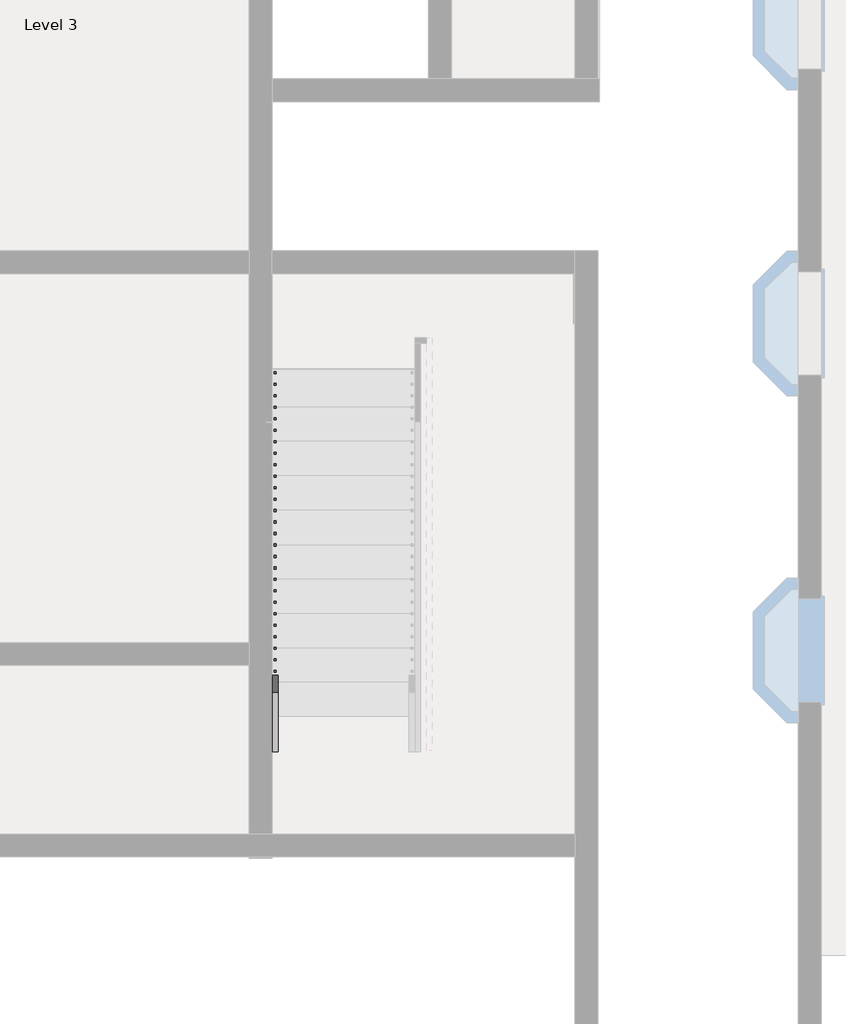
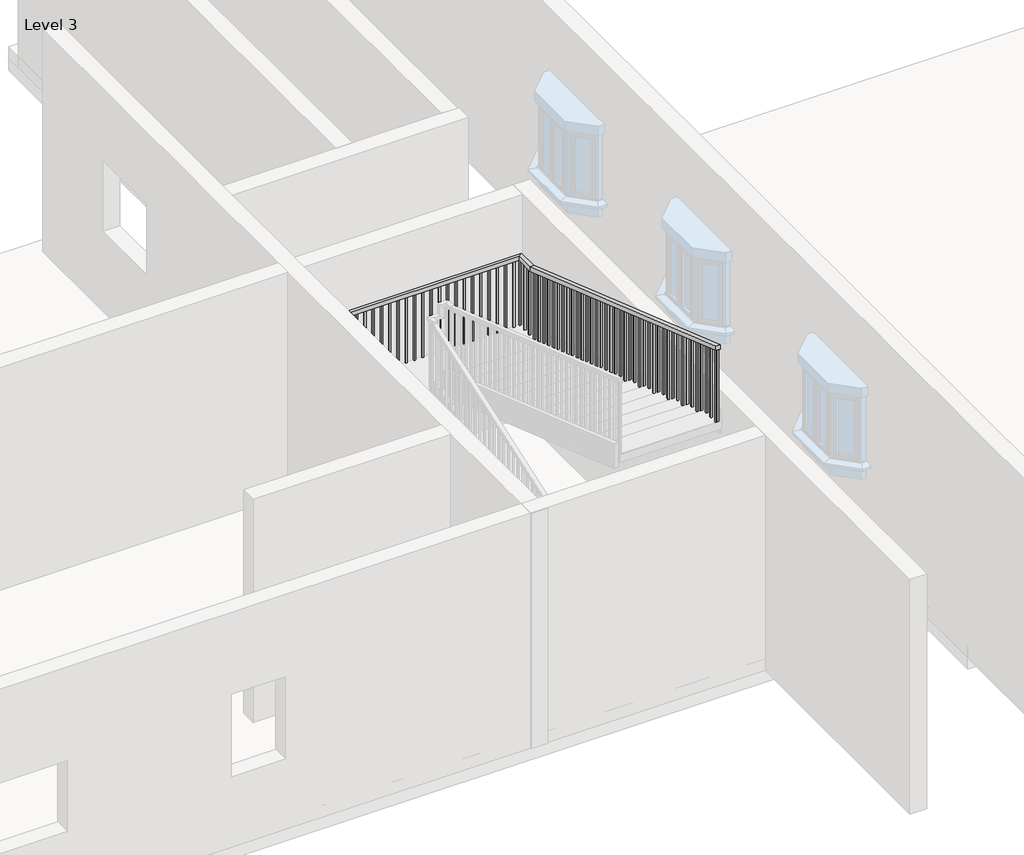
# One storey, part 8 of 14: 1 railing.
"""IFC4 building model written with IfcOpenShell, lengths in millimetres."""

from ifc_helpers import new_model, si_unit, frame, origin, place, context, project, spatial, polyline, outline, extrude, faceted_brep, element, save

model = new_model("IFC4")

# Units and contexts
model_context = context("Model", 3, world=origin())
ifc_project = project(units=[si_unit("LENGTHUNIT", "METRE", prefix="MILLI")], contexts=[model_context])

# Site, building, storey
site = spatial("IfcSite", under=ifc_project)
building = spatial("IfcBuilding", under=site)
storey = spatial("IfcBuildingStorey", under=building, Name="Level 3", Elevation=6096.0)

# Railing
placement = place(None, origin())
element("IfcRailing", 1, ObjectType="Handrail - Rectangular", at=placement, inside=storey, context=model_context, shape_type="SolidModel", body=[
    faceted_brep([(-3857.687215, -9955.5916506, 7115.9076923), (-3857.687215, -9955.5916506, 7062.1602476), (-3806.887215, -9955.5916506, 7062.1602476), (-3806.887215, -9955.5916506, 7115.9076923), (-3857.687215, -6291.6416506, 8382.0), (-3857.687215, -6283.1120276, 8331.2), (-3806.887215, -6283.1120276, 8331.2), (-3806.887215, -6291.6416506, 8382.0), (-3857.687215, -5713.7916506, 8382.0), (-3857.687215, -5713.7916506, 8331.2), (-3806.887215, -5764.5916506, 8331.2), (-3806.887215, -5764.5916506, 8382.0), (-1190.687215, -5713.7916506, 8382.0), (-1190.687215, -5713.7916506, 8331.2), (-1241.487215, -5764.5916506, 8331.2), (-1241.487215, -5764.5916506, 8382.0), (-1190.687215, -5986.8416506, 8382.0), (-1190.687215, -5995.3852679, 8331.2), (-1241.487215, -5995.3852679, 8331.2), (-1241.487215, -5986.8416506, 8382.0), (-1190.687215, -9949.2416506, 9753.6), (-1241.487215, -9949.2416506, 9753.6), (-1241.487215, -9949.2416506, 9699.842594), (-1190.687215, -9949.2416506, 9699.842594)], [[[0, 1, 2, 3]], [[1, 0, 4, 5]], [[2, 1, 5, 6]], [[3, 2, 6, 7]], [[0, 3, 7, 4]], [[5, 4, 8, 9]], [[6, 5, 9, 10]], [[7, 6, 10, 11]], [[4, 7, 11, 8]], [[9, 8, 12, 13]], [[10, 9, 13, 14]], [[11, 10, 14, 15]], [[8, 11, 15, 12]], [[13, 12, 16, 17]], [[14, 13, 17, 18]], [[15, 14, 18, 19]], [[12, 15, 19, 16]], [[20, 21, 22, 23]], [[17, 16, 20, 23]], [[18, 17, 23, 22]], [[19, 18, 22, 21]], [[16, 19, 21, 20]]]),
    extrude(outline(polyline([(-9895.2666506, 9681.1589402), (-9895.2666506, 8733.6923077), (-9914.3166506, 8733.6923077), (-9914.3166506, 9687.7531709), (-9895.2666506, 9681.1589402)])), frame((-1225.612215, 0.0, 0.0), z_axis=(1.0, 0.0, 0.0), x_axis=(0.0, 1.0, 0.0)), (0.0, 0.0, 1.0), 19.05),
    extrude(outline(polyline([(-9793.6666506, 9645.9897094), (-9793.6666506, 8733.6923077), (-9812.7166506, 8733.6923077), (-9812.7166506, 9652.5839402), (-9793.6666506, 9645.9897094)])), frame((-1225.612215, 0.0, 0.0), z_axis=(1.0, 0.0, 0.0), x_axis=(0.0, 1.0, 0.0)), (0.0, 0.0, 1.0), 19.05),
    extrude(outline(polyline([(-9692.0666506, 9610.8204786), (-9692.0666506, 8733.6923077), (-9711.1166506, 8733.6923077), (-9711.1166506, 9617.4147094), (-9692.0666506, 9610.8204786)])), frame((-1225.612215, 0.0, 0.0), z_axis=(1.0, 0.0, 0.0), x_axis=(0.0, 1.0, 0.0)), (0.0, 0.0, 1.0), 19.05),
    extrude(outline(polyline([(-9590.4666506, 9575.6512479), (-9590.4666506, 8628.1846154), (-9609.5166506, 8628.1846154), (-9609.5166506, 9582.2454786), (-9590.4666506, 9575.6512479)])), frame((-1225.612215, 0.0, 0.0), z_axis=(1.0, 0.0, 0.0), x_axis=(0.0, 1.0, 0.0)), (0.0, 0.0, 1.0), 19.05),
    extrude(outline(polyline([(-9488.8666506, 9540.4820171), (-9488.8666506, 8628.1846154), (-9507.9166506, 8628.1846154), (-9507.9166506, 9547.0762479), (-9488.8666506, 9540.4820171)])), frame((-1225.612215, 0.0, 0.0), z_axis=(1.0, 0.0, 0.0), x_axis=(0.0, 1.0, 0.0)), (0.0, 0.0, 1.0), 19.05),
    extrude(outline(polyline([(-9387.2666506, 9505.3127863), (-9387.2666506, 8628.1846154), (-9406.3166506, 8628.1846154), (-9406.3166506, 9511.9070171), (-9387.2666506, 9505.3127863)])), frame((-1225.612215, 0.0, 0.0), z_axis=(1.0, 0.0, 0.0), x_axis=(0.0, 1.0, 0.0)), (0.0, 0.0, 1.0), 19.05),
    extrude(outline(polyline([(-9285.6666506, 9470.1435556), (-9285.6666506, 8522.6769231), (-9304.7166506, 8522.6769231), (-9304.7166506, 9476.7377863), (-9285.6666506, 9470.1435556)])), frame((-1225.612215, 0.0, 0.0), z_axis=(1.0, 0.0, 0.0), x_axis=(0.0, 1.0, 0.0)), (0.0, 0.0, 1.0), 19.05),
    extrude(outline(polyline([(-9184.0666506, 9434.9743248), (-9184.0666506, 8522.6769231), (-9203.1166506, 8522.6769231), (-9203.1166506, 9441.5685556), (-9184.0666506, 9434.9743248)])), frame((-1225.612215, 0.0, 0.0), z_axis=(1.0, 0.0, 0.0), x_axis=(0.0, 1.0, 0.0)), (0.0, 0.0, 1.0), 19.05),
    extrude(outline(polyline([(-9082.4666506, 9399.805094), (-9082.4666506, 8522.6769231), (-9101.5166506, 8522.6769231), (-9101.5166506, 9406.3993248), (-9082.4666506, 9399.805094)])), frame((-1225.612215, 0.0, 0.0), z_axis=(1.0, 0.0, 0.0), x_axis=(0.0, 1.0, 0.0)), (0.0, 0.0, 1.0), 19.05),
    extrude(outline(polyline([(-8980.8666506, 9364.6358632), (-8980.8666506, 8417.1692308), (-8999.9166506, 8417.1692308), (-8999.9166506, 9371.230094), (-8980.8666506, 9364.6358632)])), frame((-1225.612215, 0.0, 0.0), z_axis=(1.0, 0.0, 0.0), x_axis=(0.0, 1.0, 0.0)), (0.0, 0.0, 1.0), 19.05),
    extrude(outline(polyline([(-8879.2666506, 9329.4666325), (-8879.2666506, 8417.1692308), (-8898.3166506, 8417.1692308), (-8898.3166506, 9336.0608632), (-8879.2666506, 9329.4666325)])), frame((-1225.612215, 0.0, 0.0), z_axis=(1.0, 0.0, 0.0), x_axis=(0.0, 1.0, 0.0)), (0.0, 0.0, 1.0), 19.05),
    extrude(outline(polyline([(-8777.6666506, 9294.2974017), (-8777.6666506, 8417.1692308), (-8796.7166506, 8417.1692308), (-8796.7166506, 9300.8916325), (-8777.6666506, 9294.2974017)])), frame((-1225.612215, 0.0, 0.0), z_axis=(1.0, 0.0, 0.0), x_axis=(0.0, 1.0, 0.0)), (0.0, 0.0, 1.0), 19.05),
    extrude(outline(polyline([(-8676.0666506, 9259.1281709), (-8676.0666506, 8311.6615385), (-8695.1166506, 8311.6615385), (-8695.1166506, 9265.7224017), (-8676.0666506, 9259.1281709)])), frame((-1225.612215, 0.0, 0.0), z_axis=(1.0, 0.0, 0.0), x_axis=(0.0, 1.0, 0.0)), (0.0, 0.0, 1.0), 19.05),
    extrude(outline(polyline([(-8574.4666506, 9223.9589402), (-8574.4666506, 8311.6615385), (-8593.5166506, 8311.6615385), (-8593.5166506, 9230.5531709), (-8574.4666506, 9223.9589402)])), frame((-1225.612215, 0.0, 0.0), z_axis=(1.0, 0.0, 0.0), x_axis=(0.0, 1.0, 0.0)), (0.0, 0.0, 1.0), 19.05),
    extrude(outline(polyline([(-8472.8666506, 9188.7897094), (-8472.8666506, 8311.6615385), (-8491.9166506, 8311.6615385), (-8491.9166506, 9195.3839402), (-8472.8666506, 9188.7897094)])), frame((-1225.612215, 0.0, 0.0), z_axis=(1.0, 0.0, 0.0), x_axis=(0.0, 1.0, 0.0)), (0.0, 0.0, 1.0), 19.05),
    extrude(outline(polyline([(-8371.2666506, 9153.6204786), (-8371.2666506, 8206.1538462), (-8390.3166506, 8206.1538462), (-8390.3166506, 9160.2147094), (-8371.2666506, 9153.6204786)])), frame((-1225.612215, 0.0, 0.0), z_axis=(1.0, 0.0, 0.0), x_axis=(0.0, 1.0, 0.0)), (0.0, 0.0, 1.0), 19.05),
    extrude(outline(polyline([(-8269.6666506, 9118.4512479), (-8269.6666506, 8206.1538462), (-8288.7166506, 8206.1538462), (-8288.7166506, 9125.0454786), (-8269.6666506, 9118.4512479)])), frame((-1225.612215, 0.0, 0.0), z_axis=(1.0, 0.0, 0.0), x_axis=(0.0, 1.0, 0.0)), (0.0, 0.0, 1.0), 19.05),
    extrude(outline(polyline([(-8168.0666506, 9083.2820171), (-8168.0666506, 8206.1538462), (-8187.1166506, 8206.1538462), (-8187.1166506, 9089.8762479), (-8168.0666506, 9083.2820171)])), frame((-1225.612215, 0.0, 0.0), z_axis=(1.0, 0.0, 0.0), x_axis=(0.0, 1.0, 0.0)), (0.0, 0.0, 1.0), 19.05),
    extrude(outline(polyline([(-8066.4666506, 9048.1127863), (-8066.4666506, 8100.6461538), (-8085.5166506, 8100.6461538), (-8085.5166506, 9054.7070171), (-8066.4666506, 9048.1127863)])), frame((-1225.612215, 0.0, 0.0), z_axis=(1.0, 0.0, 0.0), x_axis=(0.0, 1.0, 0.0)), (0.0, 0.0, 1.0), 19.05),
    extrude(outline(polyline([(-7964.8666506, 9012.9435556), (-7964.8666506, 8100.6461538), (-7983.9166506, 8100.6461538), (-7983.9166506, 9019.5377863), (-7964.8666506, 9012.9435556)])), frame((-1225.612215, 0.0, 0.0), z_axis=(1.0, 0.0, 0.0), x_axis=(0.0, 1.0, 0.0)), (0.0, 0.0, 1.0), 19.05),
    extrude(outline(polyline([(-7863.2666506, 8977.7743248), (-7863.2666506, 8100.6461538), (-7882.3166506, 8100.6461538), (-7882.3166506, 8984.3685556), (-7863.2666506, 8977.7743248)])), frame((-1225.612215, 0.0, 0.0), z_axis=(1.0, 0.0, 0.0), x_axis=(0.0, 1.0, 0.0)), (0.0, 0.0, 1.0), 19.05),
    extrude(outline(polyline([(-7761.6666506, 8942.605094), (-7761.6666506, 7995.1384615), (-7780.7166506, 7995.1384615), (-7780.7166506, 8949.1993248), (-7761.6666506, 8942.605094)])), frame((-1225.612215, 0.0, 0.0), z_axis=(1.0, 0.0, 0.0), x_axis=(0.0, 1.0, 0.0)), (0.0, 0.0, 1.0), 19.05),
    extrude(outline(polyline([(-7660.0666506, 8907.4358632), (-7660.0666506, 7995.1384615), (-7679.1166506, 7995.1384615), (-7679.1166506, 8914.030094), (-7660.0666506, 8907.4358632)])), frame((-1225.612215, 0.0, 0.0), z_axis=(1.0, 0.0, 0.0), x_axis=(0.0, 1.0, 0.0)), (0.0, 0.0, 1.0), 19.05),
    extrude(outline(polyline([(-7558.4666506, 8872.2666325), (-7558.4666506, 7995.1384615), (-7577.5166506, 7995.1384615), (-7577.5166506, 8878.8608632), (-7558.4666506, 8872.2666325)])), frame((-1225.612215, 0.0, 0.0), z_axis=(1.0, 0.0, 0.0), x_axis=(0.0, 1.0, 0.0)), (0.0, 0.0, 1.0), 19.05),
    extrude(outline(polyline([(-7456.8666506, 8837.0974017), (-7456.8666506, 7889.6307692), (-7475.9166506, 7889.6307692), (-7475.9166506, 8843.6916325), (-7456.8666506, 8837.0974017)])), frame((-1225.612215, 0.0, 0.0), z_axis=(1.0, 0.0, 0.0), x_axis=(0.0, 1.0, 0.0)), (0.0, 0.0, 1.0), 19.05),
    extrude(outline(polyline([(-7355.2666506, 8801.9281709), (-7355.2666506, 7889.6307692), (-7374.3166506, 7889.6307692), (-7374.3166506, 8808.5224017), (-7355.2666506, 8801.9281709)])), frame((-1225.612215, 0.0, 0.0), z_axis=(1.0, 0.0, 0.0), x_axis=(0.0, 1.0, 0.0)), (0.0, 0.0, 1.0), 19.05),
    extrude(outline(polyline([(-7253.6666506, 8766.7589402), (-7253.6666506, 7889.6307692), (-7272.7166506, 7889.6307692), (-7272.7166506, 8773.3531709), (-7253.6666506, 8766.7589402)])), frame((-1225.612215, 0.0, 0.0), z_axis=(1.0, 0.0, 0.0), x_axis=(0.0, 1.0, 0.0)), (0.0, 0.0, 1.0), 19.05),
    extrude(outline(polyline([(-7152.0666506, 8731.5897094), (-7152.0666506, 7784.1230769), (-7171.1166506, 7784.1230769), (-7171.1166506, 8738.1839402), (-7152.0666506, 8731.5897094)])), frame((-1225.612215, 0.0, 0.0), z_axis=(1.0, 0.0, 0.0), x_axis=(0.0, 1.0, 0.0)), (0.0, 0.0, 1.0), 19.05),
    extrude(outline(polyline([(-7050.4666506, 8696.4204786), (-7050.4666506, 7784.1230769), (-7069.5166506, 7784.1230769), (-7069.5166506, 8703.0147094), (-7050.4666506, 8696.4204786)])), frame((-1225.612215, 0.0, 0.0), z_axis=(1.0, 0.0, 0.0), x_axis=(0.0, 1.0, 0.0)), (0.0, 0.0, 1.0), 19.05),
    extrude(outline(polyline([(-6948.8666506, 8661.2512479), (-6948.8666506, 7784.1230769), (-6967.9166506, 7784.1230769), (-6967.9166506, 8667.8454786), (-6948.8666506, 8661.2512479)])), frame((-1225.612215, 0.0, 0.0), z_axis=(1.0, 0.0, 0.0), x_axis=(0.0, 1.0, 0.0)), (0.0, 0.0, 1.0), 19.05),
    extrude(outline(polyline([(-6847.2666506, 8626.0820171), (-6847.2666506, 7678.6153846), (-6866.3166506, 7678.6153846), (-6866.3166506, 8632.6762479), (-6847.2666506, 8626.0820171)])), frame((-1225.612215, 0.0, 0.0), z_axis=(1.0, 0.0, 0.0), x_axis=(0.0, 1.0, 0.0)), (0.0, 0.0, 1.0), 19.05),
    extrude(outline(polyline([(-6745.6666506, 8590.9127863), (-6745.6666506, 7678.6153846), (-6764.7166506, 7678.6153846), (-6764.7166506, 8597.5070171), (-6745.6666506, 8590.9127863)])), frame((-1225.612215, 0.0, 0.0), z_axis=(1.0, 0.0, 0.0), x_axis=(0.0, 1.0, 0.0)), (0.0, 0.0, 1.0), 19.05),
    extrude(outline(polyline([(-6644.0666506, 8555.7435556), (-6644.0666506, 7678.6153846), (-6663.1166506, 7678.6153846), (-6663.1166506, 8562.3377863), (-6644.0666506, 8555.7435556)])), frame((-1225.612215, 0.0, 0.0), z_axis=(1.0, 0.0, 0.0), x_axis=(0.0, 1.0, 0.0)), (0.0, 0.0, 1.0), 19.05),
    extrude(outline(polyline([(-6542.4666506, 8520.5743248), (-6542.4666506, 7573.1076923), (-6561.5166506, 7573.1076923), (-6561.5166506, 8527.1685556), (-6542.4666506, 8520.5743248)])), frame((-1225.612215, 0.0, 0.0), z_axis=(1.0, 0.0, 0.0), x_axis=(0.0, 1.0, 0.0)), (0.0, 0.0, 1.0), 19.05),
    extrude(outline(polyline([(-6440.8666506, 8485.405094), (-6440.8666506, 7573.1076923), (-6459.9166506, 7573.1076923), (-6459.9166506, 8491.9993248), (-6440.8666506, 8485.405094)])), frame((-1225.612215, 0.0, 0.0), z_axis=(1.0, 0.0, 0.0), x_axis=(0.0, 1.0, 0.0)), (0.0, 0.0, 1.0), 19.05),
    extrude(outline(polyline([(-6339.2666506, 8450.2358632), (-6339.2666506, 7573.1076923), (-6358.3166506, 7573.1076923), (-6358.3166506, 8456.830094), (-6339.2666506, 8450.2358632)])), frame((-1225.612215, 0.0, 0.0), z_axis=(1.0, 0.0, 0.0), x_axis=(0.0, 1.0, 0.0)), (0.0, 0.0, 1.0), 19.05),
    extrude(outline(polyline([(-6237.6666506, 8415.0666325), (-6237.6666506, 7467.6), (-6256.7166506, 7467.6), (-6256.7166506, 8421.6608632), (-6237.6666506, 8415.0666325)])), frame((-1225.612215, 0.0, 0.0), z_axis=(1.0, 0.0, 0.0), x_axis=(0.0, 1.0, 0.0)), (0.0, 0.0, 1.0), 19.05),
    extrude(outline(polyline([(-6136.0666506, 8379.8974017), (-6136.0666506, 7467.6), (-6155.1166506, 7467.6), (-6155.1166506, 8386.4916325), (-6136.0666506, 8379.8974017)])), frame((-1225.612215, 0.0, 0.0), z_axis=(1.0, 0.0, 0.0), x_axis=(0.0, 1.0, 0.0)), (0.0, 0.0, 1.0), 19.05),
    extrude(outline(polyline([(-6034.4666506, 8344.7281709), (-6034.4666506, 7467.6), (-6053.5166506, 7467.6), (-6053.5166506, 8351.3224017), (-6034.4666506, 8344.7281709)])), frame((-1225.612215, 0.0, 0.0), z_axis=(1.0, 0.0, 0.0), x_axis=(0.0, 1.0, 0.0)), (0.0, 0.0, 1.0), 19.05),
    extrude(outline(polyline([(-1206.562215, -5932.8666506), (-1206.562215, -5951.9166506), (-1225.612215, -5951.9166506), (-1225.612215, -5932.8666506), (-1206.562215, -5932.8666506)])), frame((0.0, 0.0, 7467.6), z_axis=(0.0, 0.0, 1.0), x_axis=(1.0, 0.0, 0.0)), (0.0, 0.0, 1.0), 863.6),
    extrude(outline(polyline([(-1206.562215, -5831.2666506), (-1206.562215, -5850.3166506), (-1225.612215, -5850.3166506), (-1225.612215, -5831.2666506), (-1206.562215, -5831.2666506)])), frame((0.0, 0.0, 7467.6), z_axis=(0.0, 0.0, 1.0), x_axis=(1.0, 0.0, 0.0)), (0.0, 0.0, 1.0), 863.6),
    extrude(outline(polyline([(-1301.812215, -5729.6666506), (-1282.762215, -5729.6666506), (-1282.762215, -5748.7166506), (-1301.812215, -5748.7166506), (-1301.812215, -5729.6666506)])), frame((0.0, 0.0, 7467.6), z_axis=(0.0, 0.0, 1.0), x_axis=(1.0, 0.0, 0.0)), (0.0, 0.0, 1.0), 863.6),
    extrude(outline(polyline([(-1403.412215, -5729.6666506), (-1384.362215, -5729.6666506), (-1384.362215, -5748.7166506), (-1403.412215, -5748.7166506), (-1403.412215, -5729.6666506)])), frame((0.0, 0.0, 7467.6), z_axis=(0.0, 0.0, 1.0), x_axis=(1.0, 0.0, 0.0)), (0.0, 0.0, 1.0), 863.6),
    extrude(outline(polyline([(-1505.012215, -5729.6666506), (-1485.962215, -5729.6666506), (-1485.962215, -5748.7166506), (-1505.012215, -5748.7166506), (-1505.012215, -5729.6666506)])), frame((0.0, 0.0, 7467.6), z_axis=(0.0, 0.0, 1.0), x_axis=(1.0, 0.0, 0.0)), (0.0, 0.0, 1.0), 863.6),
    extrude(outline(polyline([(-1606.612215, -5729.6666506), (-1587.562215, -5729.6666506), (-1587.562215, -5748.7166506), (-1606.612215, -5748.7166506), (-1606.612215, -5729.6666506)])), frame((0.0, 0.0, 7467.6), z_axis=(0.0, 0.0, 1.0), x_axis=(1.0, 0.0, 0.0)), (0.0, 0.0, 1.0), 863.6),
    extrude(outline(polyline([(-1708.212215, -5729.6666506), (-1689.162215, -5729.6666506), (-1689.162215, -5748.7166506), (-1708.212215, -5748.7166506), (-1708.212215, -5729.6666506)])), frame((0.0, 0.0, 7467.6), z_axis=(0.0, 0.0, 1.0), x_axis=(1.0, 0.0, 0.0)), (0.0, 0.0, 1.0), 863.6),
    extrude(outline(polyline([(-1809.812215, -5729.6666506), (-1790.762215, -5729.6666506), (-1790.762215, -5748.7166506), (-1809.812215, -5748.7166506), (-1809.812215, -5729.6666506)])), frame((0.0, 0.0, 7467.6), z_axis=(0.0, 0.0, 1.0), x_axis=(1.0, 0.0, 0.0)), (0.0, 0.0, 1.0), 863.6),
    extrude(outline(polyline([(-1911.412215, -5729.6666506), (-1892.362215, -5729.6666506), (-1892.362215, -5748.7166506), (-1911.412215, -5748.7166506), (-1911.412215, -5729.6666506)])), frame((0.0, 0.0, 7467.6), z_axis=(0.0, 0.0, 1.0), x_axis=(1.0, 0.0, 0.0)), (0.0, 0.0, 1.0), 863.6),
    extrude(outline(polyline([(-2013.012215, -5729.6666506), (-1993.962215, -5729.6666506), (-1993.962215, -5748.7166506), (-2013.012215, -5748.7166506), (-2013.012215, -5729.6666506)])), frame((0.0, 0.0, 7467.6), z_axis=(0.0, 0.0, 1.0), x_axis=(1.0, 0.0, 0.0)), (0.0, 0.0, 1.0), 863.6),
    extrude(outline(polyline([(-2114.612215, -5729.6666506), (-2095.562215, -5729.6666506), (-2095.562215, -5748.7166506), (-2114.612215, -5748.7166506), (-2114.612215, -5729.6666506)])), frame((0.0, 0.0, 7467.6), z_axis=(0.0, 0.0, 1.0), x_axis=(1.0, 0.0, 0.0)), (0.0, 0.0, 1.0), 863.6),
    extrude(outline(polyline([(-2216.212215, -5729.6666506), (-2197.162215, -5729.6666506), (-2197.162215, -5748.7166506), (-2216.212215, -5748.7166506), (-2216.212215, -5729.6666506)])), frame((0.0, 0.0, 7467.6), z_axis=(0.0, 0.0, 1.0), x_axis=(1.0, 0.0, 0.0)), (0.0, 0.0, 1.0), 863.6),
    extrude(outline(polyline([(-2317.812215, -5729.6666506), (-2298.762215, -5729.6666506), (-2298.762215, -5748.7166506), (-2317.812215, -5748.7166506), (-2317.812215, -5729.6666506)])), frame((0.0, 0.0, 7467.6), z_axis=(0.0, 0.0, 1.0), x_axis=(1.0, 0.0, 0.0)), (0.0, 0.0, 1.0), 863.6),
    extrude(outline(polyline([(-2419.412215, -5729.6666506), (-2400.362215, -5729.6666506), (-2400.362215, -5748.7166506), (-2419.412215, -5748.7166506), (-2419.412215, -5729.6666506)])), frame((0.0, 0.0, 7467.6), z_axis=(0.0, 0.0, 1.0), x_axis=(1.0, 0.0, 0.0)), (0.0, 0.0, 1.0), 863.6),
    extrude(outline(polyline([(-2521.012215, -5729.6666506), (-2501.962215, -5729.6666506), (-2501.962215, -5748.7166506), (-2521.012215, -5748.7166506), (-2521.012215, -5729.6666506)])), frame((0.0, 0.0, 7467.6), z_axis=(0.0, 0.0, 1.0), x_axis=(1.0, 0.0, 0.0)), (0.0, 0.0, 1.0), 863.6),
    extrude(outline(polyline([(-2622.612215, -5729.6666506), (-2603.562215, -5729.6666506), (-2603.562215, -5748.7166506), (-2622.612215, -5748.7166506), (-2622.612215, -5729.6666506)])), frame((0.0, 0.0, 7467.6), z_axis=(0.0, 0.0, 1.0), x_axis=(1.0, 0.0, 0.0)), (0.0, 0.0, 1.0), 863.6),
    extrude(outline(polyline([(-2724.212215, -5729.6666506), (-2705.162215, -5729.6666506), (-2705.162215, -5748.7166506), (-2724.212215, -5748.7166506), (-2724.212215, -5729.6666506)])), frame((0.0, 0.0, 7467.6), z_axis=(0.0, 0.0, 1.0), x_axis=(1.0, 0.0, 0.0)), (0.0, 0.0, 1.0), 863.6),
    extrude(outline(polyline([(-2825.812215, -5729.6666506), (-2806.762215, -5729.6666506), (-2806.762215, -5748.7166506), (-2825.812215, -5748.7166506), (-2825.812215, -5729.6666506)])), frame((0.0, 0.0, 7467.6), z_axis=(0.0, 0.0, 1.0), x_axis=(1.0, 0.0, 0.0)), (0.0, 0.0, 1.0), 863.6),
    extrude(outline(polyline([(-2927.412215, -5729.6666506), (-2908.362215, -5729.6666506), (-2908.362215, -5748.7166506), (-2927.412215, -5748.7166506), (-2927.412215, -5729.6666506)])), frame((0.0, 0.0, 7467.6), z_axis=(0.0, 0.0, 1.0), x_axis=(1.0, 0.0, 0.0)), (0.0, 0.0, 1.0), 863.6),
    extrude(outline(polyline([(-3029.012215, -5729.6666506), (-3009.962215, -5729.6666506), (-3009.962215, -5748.7166506), (-3029.012215, -5748.7166506), (-3029.012215, -5729.6666506)])), frame((0.0, 0.0, 7467.6), z_axis=(0.0, 0.0, 1.0), x_axis=(1.0, 0.0, 0.0)), (0.0, 0.0, 1.0), 863.6),
    extrude(outline(polyline([(-3130.612215, -5729.6666506), (-3111.562215, -5729.6666506), (-3111.562215, -5748.7166506), (-3130.612215, -5748.7166506), (-3130.612215, -5729.6666506)])), frame((0.0, 0.0, 7467.6), z_axis=(0.0, 0.0, 1.0), x_axis=(1.0, 0.0, 0.0)), (0.0, 0.0, 1.0), 863.6),
    extrude(outline(polyline([(-3232.212215, -5729.6666506), (-3213.162215, -5729.6666506), (-3213.162215, -5748.7166506), (-3232.212215, -5748.7166506), (-3232.212215, -5729.6666506)])), frame((0.0, 0.0, 7467.6), z_axis=(0.0, 0.0, 1.0), x_axis=(1.0, 0.0, 0.0)), (0.0, 0.0, 1.0), 863.6),
    extrude(outline(polyline([(-3333.812215, -5729.6666506), (-3314.762215, -5729.6666506), (-3314.762215, -5748.7166506), (-3333.812215, -5748.7166506), (-3333.812215, -5729.6666506)])), frame((0.0, 0.0, 7467.6), z_axis=(0.0, 0.0, 1.0), x_axis=(1.0, 0.0, 0.0)), (0.0, 0.0, 1.0), 863.6),
    extrude(outline(polyline([(-3435.412215, -5729.6666506), (-3416.362215, -5729.6666506), (-3416.362215, -5748.7166506), (-3435.412215, -5748.7166506), (-3435.412215, -5729.6666506)])), frame((0.0, 0.0, 7467.6), z_axis=(0.0, 0.0, 1.0), x_axis=(1.0, 0.0, 0.0)), (0.0, 0.0, 1.0), 863.6),
    extrude(outline(polyline([(-3537.012215, -5729.6666506), (-3517.962215, -5729.6666506), (-3517.962215, -5748.7166506), (-3537.012215, -5748.7166506), (-3537.012215, -5729.6666506)])), frame((0.0, 0.0, 7467.6), z_axis=(0.0, 0.0, 1.0), x_axis=(1.0, 0.0, 0.0)), (0.0, 0.0, 1.0), 863.6),
    extrude(outline(polyline([(-3638.612215, -5729.6666506), (-3619.562215, -5729.6666506), (-3619.562215, -5748.7166506), (-3638.612215, -5748.7166506), (-3638.612215, -5729.6666506)])), frame((0.0, 0.0, 7467.6), z_axis=(0.0, 0.0, 1.0), x_axis=(1.0, 0.0, 0.0)), (0.0, 0.0, 1.0), 863.6),
    extrude(outline(polyline([(-3740.212215, -5729.6666506), (-3721.162215, -5729.6666506), (-3721.162215, -5748.7166506), (-3740.212215, -5748.7166506), (-3740.212215, -5729.6666506)])), frame((0.0, 0.0, 7467.6), z_axis=(0.0, 0.0, 1.0), x_axis=(1.0, 0.0, 0.0)), (0.0, 0.0, 1.0), 863.6),
    extrude(outline(polyline([(-3841.812215, -5799.5166506), (-3841.812215, -5780.4666506), (-3822.762215, -5780.4666506), (-3822.762215, -5799.5166506), (-3841.812215, -5799.5166506)])), frame((0.0, 0.0, 7467.6), z_axis=(0.0, 0.0, 1.0), x_axis=(1.0, 0.0, 0.0)), (0.0, 0.0, 1.0), 863.6),
    extrude(outline(polyline([(-3841.812215, -5901.1166506), (-3841.812215, -5882.0666506), (-3822.762215, -5882.0666506), (-3822.762215, -5901.1166506), (-3841.812215, -5901.1166506)])), frame((0.0, 0.0, 7467.6), z_axis=(0.0, 0.0, 1.0), x_axis=(1.0, 0.0, 0.0)), (0.0, 0.0, 1.0), 863.6),
    extrude(outline(polyline([(-3841.812215, -6002.7166506), (-3841.812215, -5983.6666506), (-3822.762215, -5983.6666506), (-3822.762215, -6002.7166506), (-3841.812215, -6002.7166506)])), frame((0.0, 0.0, 7467.6), z_axis=(0.0, 0.0, 1.0), x_axis=(1.0, 0.0, 0.0)), (0.0, 0.0, 1.0), 863.6),
    extrude(outline(polyline([(-3841.812215, -6104.3166506), (-3841.812215, -6085.2666506), (-3822.762215, -6085.2666506), (-3822.762215, -6104.3166506), (-3841.812215, -6104.3166506)])), frame((0.0, 0.0, 7467.6), z_axis=(0.0, 0.0, 1.0), x_axis=(1.0, 0.0, 0.0)), (0.0, 0.0, 1.0), 863.6),
    extrude(outline(polyline([(-3841.812215, -6205.9166506), (-3841.812215, -6186.8666506), (-3822.762215, -6186.8666506), (-3822.762215, -6205.9166506), (-3841.812215, -6205.9166506)])), frame((0.0, 0.0, 7467.6), z_axis=(0.0, 0.0, 1.0), x_axis=(1.0, 0.0, 0.0)), (0.0, 0.0, 1.0), 863.6),
    extrude(outline(polyline([(-6288.4666506, 8329.349689), (-6288.4666506, 7362.0923077), (-6307.5166506, 7362.0923077), (-6307.5166506, 8322.7668867), (-6288.4666506, 8329.349689)])), frame((-3841.812215, 0.0, 0.0), z_axis=(1.0, 0.0, 0.0), x_axis=(0.0, 1.0, 0.0)), (0.0, 0.0, 1.0), 19.05),
    extrude(outline(polyline([(-6390.0666506, 8294.2414101), (-6390.0666506, 7362.0923077), (-6409.1166506, 7362.0923077), (-6409.1166506, 8287.6586078), (-6390.0666506, 8294.2414101)])), frame((-3841.812215, 0.0, 0.0), z_axis=(1.0, 0.0, 0.0), x_axis=(0.0, 1.0, 0.0)), (0.0, 0.0, 1.0), 19.05),
    extrude(outline(polyline([(-6491.6666506, 8259.1331312), (-6491.6666506, 7362.0923077), (-6510.7166506, 7362.0923077), (-6510.7166506, 8252.5503289), (-6491.6666506, 8259.1331312)])), frame((-3841.812215, 0.0, 0.0), z_axis=(1.0, 0.0, 0.0), x_axis=(0.0, 1.0, 0.0)), (0.0, 0.0, 1.0), 19.05),
    extrude(outline(polyline([(-6593.2666506, 8224.0248523), (-6593.2666506, 7256.5846154), (-6612.3166506, 7256.5846154), (-6612.3166506, 8217.44205), (-6593.2666506, 8224.0248523)])), frame((-3841.812215, 0.0, 0.0), z_axis=(1.0, 0.0, 0.0), x_axis=(0.0, 1.0, 0.0)), (0.0, 0.0, 1.0), 19.05),
    extrude(outline(polyline([(-6694.8666506, 8188.9165734), (-6694.8666506, 7256.5846154), (-6713.9166506, 7256.5846154), (-6713.9166506, 8182.3337711), (-6694.8666506, 8188.9165734)])), frame((-3841.812215, 0.0, 0.0), z_axis=(1.0, 0.0, 0.0), x_axis=(0.0, 1.0, 0.0)), (0.0, 0.0, 1.0), 19.05),
    extrude(outline(polyline([(-6796.4666506, 8153.8082945), (-6796.4666506, 7256.5846154), (-6815.5166506, 7256.5846154), (-6815.5166506, 8147.2254922), (-6796.4666506, 8153.8082945)])), frame((-3841.812215, 0.0, 0.0), z_axis=(1.0, 0.0, 0.0), x_axis=(0.0, 1.0, 0.0)), (0.0, 0.0, 1.0), 19.05),
    extrude(outline(polyline([(-6898.0666506, 8118.7000156), (-6898.0666506, 7151.0769231), (-6917.1166506, 7151.0769231), (-6917.1166506, 8112.1172133), (-6898.0666506, 8118.7000156)])), frame((-3841.812215, 0.0, 0.0), z_axis=(1.0, 0.0, 0.0), x_axis=(0.0, 1.0, 0.0)), (0.0, 0.0, 1.0), 19.05),
    extrude(outline(polyline([(-6999.6666506, 8083.5917367), (-6999.6666506, 7151.0769231), (-7018.7166506, 7151.0769231), (-7018.7166506, 8077.0089344), (-6999.6666506, 8083.5917367)])), frame((-3841.812215, 0.0, 0.0), z_axis=(1.0, 0.0, 0.0), x_axis=(0.0, 1.0, 0.0)), (0.0, 0.0, 1.0), 19.05),
    extrude(outline(polyline([(-7101.2666506, 8048.4834578), (-7101.2666506, 7151.0769231), (-7120.3166506, 7151.0769231), (-7120.3166506, 8041.9006556), (-7101.2666506, 8048.4834578)])), frame((-3841.812215, 0.0, 0.0), z_axis=(1.0, 0.0, 0.0), x_axis=(0.0, 1.0, 0.0)), (0.0, 0.0, 1.0), 19.05),
    extrude(outline(polyline([(-7202.8666506, 8013.3751789), (-7202.8666506, 7045.5692308), (-7221.9166506, 7045.5692308), (-7221.9166506, 8006.7923767), (-7202.8666506, 8013.3751789)])), frame((-3841.812215, 0.0, 0.0), z_axis=(1.0, 0.0, 0.0), x_axis=(0.0, 1.0, 0.0)), (0.0, 0.0, 1.0), 19.05),
    extrude(outline(polyline([(-7304.4666506, 7978.2669001), (-7304.4666506, 7045.5692308), (-7323.5166506, 7045.5692308), (-7323.5166506, 7971.6840978), (-7304.4666506, 7978.2669001)])), frame((-3841.812215, 0.0, 0.0), z_axis=(1.0, 0.0, 0.0), x_axis=(0.0, 1.0, 0.0)), (0.0, 0.0, 1.0), 19.05),
    extrude(outline(polyline([(-7406.0666506, 7943.1586212), (-7406.0666506, 7045.5692308), (-7425.1166506, 7045.5692308), (-7425.1166506, 7936.5758189), (-7406.0666506, 7943.1586212)])), frame((-3841.812215, 0.0, 0.0), z_axis=(1.0, 0.0, 0.0), x_axis=(0.0, 1.0, 0.0)), (0.0, 0.0, 1.0), 19.05),
    extrude(outline(polyline([(-7507.6666506, 7908.0503423), (-7507.6666506, 6940.0615385), (-7526.7166506, 6940.0615385), (-7526.7166506, 7901.46754), (-7507.6666506, 7908.0503423)])), frame((-3841.812215, 0.0, 0.0), z_axis=(1.0, 0.0, 0.0), x_axis=(0.0, 1.0, 0.0)), (0.0, 0.0, 1.0), 19.05),
    extrude(outline(polyline([(-7609.2666506, 7872.9420634), (-7609.2666506, 6940.0615385), (-7628.3166506, 6940.0615385), (-7628.3166506, 7866.3592611), (-7609.2666506, 7872.9420634)])), frame((-3841.812215, 0.0, 0.0), z_axis=(1.0, 0.0, 0.0), x_axis=(0.0, 1.0, 0.0)), (0.0, 0.0, 1.0), 19.05),
    extrude(outline(polyline([(-7710.8666506, 7837.8337845), (-7710.8666506, 6940.0615385), (-7729.9166506, 6940.0615385), (-7729.9166506, 7831.2509822), (-7710.8666506, 7837.8337845)])), frame((-3841.812215, 0.0, 0.0), z_axis=(1.0, 0.0, 0.0), x_axis=(0.0, 1.0, 0.0)), (0.0, 0.0, 1.0), 19.05),
    extrude(outline(polyline([(-7812.4666506, 7802.7255056), (-7812.4666506, 6834.5538462), (-7831.5166506, 6834.5538462), (-7831.5166506, 7796.1427033), (-7812.4666506, 7802.7255056)])), frame((-3841.812215, 0.0, 0.0), z_axis=(1.0, 0.0, 0.0), x_axis=(0.0, 1.0, 0.0)), (0.0, 0.0, 1.0), 19.05),
    extrude(outline(polyline([(-7914.0666506, 7767.6172267), (-7914.0666506, 6834.5538462), (-7933.1166506, 6834.5538462), (-7933.1166506, 7761.0344244), (-7914.0666506, 7767.6172267)])), frame((-3841.812215, 0.0, 0.0), z_axis=(1.0, 0.0, 0.0), x_axis=(0.0, 1.0, 0.0)), (0.0, 0.0, 1.0), 19.05),
    extrude(outline(polyline([(-8015.6666506, 7732.5089478), (-8015.6666506, 6834.5538462), (-8034.7166506, 6834.5538462), (-8034.7166506, 7725.9261455), (-8015.6666506, 7732.5089478)])), frame((-3841.812215, 0.0, 0.0), z_axis=(1.0, 0.0, 0.0), x_axis=(0.0, 1.0, 0.0)), (0.0, 0.0, 1.0), 19.05),
    extrude(outline(polyline([(-8117.2666506, 7697.4006689), (-8117.2666506, 6729.0461538), (-8136.3166506, 6729.0461538), (-8136.3166506, 7690.8178666), (-8117.2666506, 7697.4006689)])), frame((-3841.812215, 0.0, 0.0), z_axis=(1.0, 0.0, 0.0), x_axis=(0.0, 1.0, 0.0)), (0.0, 0.0, 1.0), 19.05),
    extrude(outline(polyline([(-8218.8666506, 7662.29239), (-8218.8666506, 6729.0461538), (-8237.9166506, 6729.0461538), (-8237.9166506, 7655.7095877), (-8218.8666506, 7662.29239)])), frame((-3841.812215, 0.0, 0.0), z_axis=(1.0, 0.0, 0.0), x_axis=(0.0, 1.0, 0.0)), (0.0, 0.0, 1.0), 19.05),
    extrude(outline(polyline([(-8320.4666506, 7627.1841111), (-8320.4666506, 6729.0461538), (-8339.5166506, 6729.0461538), (-8339.5166506, 7620.6013088), (-8320.4666506, 7627.1841111)])), frame((-3841.812215, 0.0, 0.0), z_axis=(1.0, 0.0, 0.0), x_axis=(0.0, 1.0, 0.0)), (0.0, 0.0, 1.0), 19.05),
    extrude(outline(polyline([(-8422.0666506, 7592.0758322), (-8422.0666506, 6623.5384615), (-8441.1166506, 6623.5384615), (-8441.1166506, 7585.4930299), (-8422.0666506, 7592.0758322)])), frame((-3841.812215, 0.0, 0.0), z_axis=(1.0, 0.0, 0.0), x_axis=(0.0, 1.0, 0.0)), (0.0, 0.0, 1.0), 19.05),
    extrude(outline(polyline([(-8523.6666506, 7556.9675533), (-8523.6666506, 6623.5384615), (-8542.7166506, 6623.5384615), (-8542.7166506, 7550.384751), (-8523.6666506, 7556.9675533)])), frame((-3841.812215, 0.0, 0.0), z_axis=(1.0, 0.0, 0.0), x_axis=(0.0, 1.0, 0.0)), (0.0, 0.0, 1.0), 19.05),
    extrude(outline(polyline([(-8625.2666506, 7521.8592744), (-8625.2666506, 6623.5384615), (-8644.3166506, 6623.5384615), (-8644.3166506, 7515.2764721), (-8625.2666506, 7521.8592744)])), frame((-3841.812215, 0.0, 0.0), z_axis=(1.0, 0.0, 0.0), x_axis=(0.0, 1.0, 0.0)), (0.0, 0.0, 1.0), 19.05),
    extrude(outline(polyline([(-8726.8666506, 7486.7509955), (-8726.8666506, 6518.0307692), (-8745.9166506, 6518.0307692), (-8745.9166506, 7480.1681932), (-8726.8666506, 7486.7509955)])), frame((-3841.812215, 0.0, 0.0), z_axis=(1.0, 0.0, 0.0), x_axis=(0.0, 1.0, 0.0)), (0.0, 0.0, 1.0), 19.05),
    extrude(outline(polyline([(-8828.4666506, 7451.6427166), (-8828.4666506, 6518.0307692), (-8847.5166506, 6518.0307692), (-8847.5166506, 7445.0599143), (-8828.4666506, 7451.6427166)])), frame((-3841.812215, 0.0, 0.0), z_axis=(1.0, 0.0, 0.0), x_axis=(0.0, 1.0, 0.0)), (0.0, 0.0, 1.0), 19.05),
    extrude(outline(polyline([(-8930.0666506, 7416.5344377), (-8930.0666506, 6518.0307692), (-8949.1166506, 6518.0307692), (-8949.1166506, 7409.9516354), (-8930.0666506, 7416.5344377)])), frame((-3841.812215, 0.0, 0.0), z_axis=(1.0, 0.0, 0.0), x_axis=(0.0, 1.0, 0.0)), (0.0, 0.0, 1.0), 19.05),
    extrude(outline(polyline([(-9031.6666506, 7381.4261588), (-9031.6666506, 6412.5230769), (-9050.7166506, 6412.5230769), (-9050.7166506, 7374.8433565), (-9031.6666506, 7381.4261588)])), frame((-3841.812215, 0.0, 0.0), z_axis=(1.0, 0.0, 0.0), x_axis=(0.0, 1.0, 0.0)), (0.0, 0.0, 1.0), 19.05),
    extrude(outline(polyline([(-9133.2666506, 7346.3178799), (-9133.2666506, 6412.5230769), (-9152.3166506, 6412.5230769), (-9152.3166506, 7339.7350776), (-9133.2666506, 7346.3178799)])), frame((-3841.812215, 0.0, 0.0), z_axis=(1.0, 0.0, 0.0), x_axis=(0.0, 1.0, 0.0)), (0.0, 0.0, 1.0), 19.05),
    extrude(outline(polyline([(-9234.8666506, 7311.209601), (-9234.8666506, 6412.5230769), (-9253.9166506, 6412.5230769), (-9253.9166506, 7304.6267987), (-9234.8666506, 7311.209601)])), frame((-3841.812215, 0.0, 0.0), z_axis=(1.0, 0.0, 0.0), x_axis=(0.0, 1.0, 0.0)), (0.0, 0.0, 1.0), 19.05),
    extrude(outline(polyline([(-9336.4666506, 7276.1013221), (-9336.4666506, 6307.0153846), (-9355.5166506, 6307.0153846), (-9355.5166506, 7269.5185198), (-9336.4666506, 7276.1013221)])), frame((-3841.812215, 0.0, 0.0), z_axis=(1.0, 0.0, 0.0), x_axis=(0.0, 1.0, 0.0)), (0.0, 0.0, 1.0), 19.05),
    extrude(outline(polyline([(-9438.0666506, 7240.9930432), (-9438.0666506, 6307.0153846), (-9457.1166506, 6307.0153846), (-9457.1166506, 7234.4102409), (-9438.0666506, 7240.9930432)])), frame((-3841.812215, 0.0, 0.0), z_axis=(1.0, 0.0, 0.0), x_axis=(0.0, 1.0, 0.0)), (0.0, 0.0, 1.0), 19.05),
    extrude(outline(polyline([(-9539.6666506, 7205.8847643), (-9539.6666506, 6307.0153846), (-9558.7166506, 6307.0153846), (-9558.7166506, 7199.301962), (-9539.6666506, 7205.8847643)])), frame((-3841.812215, 0.0, 0.0), z_axis=(1.0, 0.0, 0.0), x_axis=(0.0, 1.0, 0.0)), (0.0, 0.0, 1.0), 19.05),
    extrude(outline(polyline([(-9641.2666506, 7170.7764854), (-9641.2666506, 6201.5076923), (-9660.3166506, 6201.5076923), (-9660.3166506, 7164.1936831), (-9641.2666506, 7170.7764854)])), frame((-3841.812215, 0.0, 0.0), z_axis=(1.0, 0.0, 0.0), x_axis=(0.0, 1.0, 0.0)), (0.0, 0.0, 1.0), 19.05),
    extrude(outline(polyline([(-9742.8666506, 7135.6682065), (-9742.8666506, 6201.5076923), (-9761.9166506, 6201.5076923), (-9761.9166506, 7129.0854043), (-9742.8666506, 7135.6682065)])), frame((-3841.812215, 0.0, 0.0), z_axis=(1.0, 0.0, 0.0), x_axis=(0.0, 1.0, 0.0)), (0.0, 0.0, 1.0), 19.05),
    extrude(outline(polyline([(-9844.4666506, 7100.5599277), (-9844.4666506, 6201.5076923), (-9863.5166506, 6201.5076923), (-9863.5166506, 7093.9771254), (-9844.4666506, 7100.5599277)])), frame((-3841.812215, 0.0, 0.0), z_axis=(1.0, 0.0, 0.0), x_axis=(0.0, 1.0, 0.0)), (0.0, 0.0, 1.0), 19.05),
    extrude(outline(polyline([(-1225.612215, -5729.6666506), (-1206.562215, -5729.6666506), (-1206.562215, -5748.7166506), (-1225.612215, -5748.7166506), (-1225.612215, -5729.6666506)])), frame((0.0, 0.0, 7467.6), z_axis=(0.0, 0.0, 1.0), x_axis=(1.0, 0.0, 0.0)), (0.0, 0.0, 1.0), 863.6),
    extrude(outline(polyline([(-3841.812215, -5748.7166506), (-3841.812215, -5729.6666506), (-3822.762215, -5729.6666506), (-3822.762215, -5748.7166506), (-3841.812215, -5748.7166506)])), frame((0.0, 0.0, 7467.6), z_axis=(0.0, 0.0, 1.0), x_axis=(1.0, 0.0, 0.0)), (0.0, 0.0, 1.0), 863.6),
    extrude(outline(polyline([(-9930.1916506, 9693.2483632), (-9930.1916506, 8733.6923077), (-9949.2416506, 8733.6923077), (-9949.2416506, 9699.842594), (-9930.1916506, 9693.2483632)])), frame((-1225.612215, 0.0, 0.0), z_axis=(1.0, 0.0, 0.0), x_axis=(0.0, 1.0, 0.0)), (0.0, 0.0, 1.0), 19.05),
    extrude(outline(polyline([(-9936.5416506, 7068.7430499), (-9936.5416506, 6201.5076923), (-9955.5916506, 6201.5076923), (-9955.5916506, 7062.1602476), (-9936.5416506, 7068.7430499)])), frame((-3841.812215, 0.0, 0.0), z_axis=(1.0, 0.0, 0.0), x_axis=(0.0, 1.0, 0.0)), (0.0, 0.0, 1.0), 19.05),
])

save(model, "model.ifc")

# Revit data of these elements
# Type "Handrail - Rectangular"
#   Assembly Code = "C2010400"
#   built-in parameter 1008612 = 0.0416667 (stored number, unit not read)
#   built-in parameter 1008611 = 0.0416667 (stored number, unit not read)
#   built-in parameter 1008609 = 0.333333 (stored number, unit not read)
#   built-in parameter 1008604 = 0.166667 (stored number, unit not read)
#   built-in parameter 1008603 = 0.166667 (stored number, unit not read)
#   Railing Height = 3' - 0"
#   built-in parameter 1008630 = 2
#   built-in parameter 1008610 = 2
#   built-in parameter 1008618 = Baluster - Square : 3/4"
# Element 1 (IfcRailing, "Handrail - Rectangular")
#   Phase Created = New Construction
